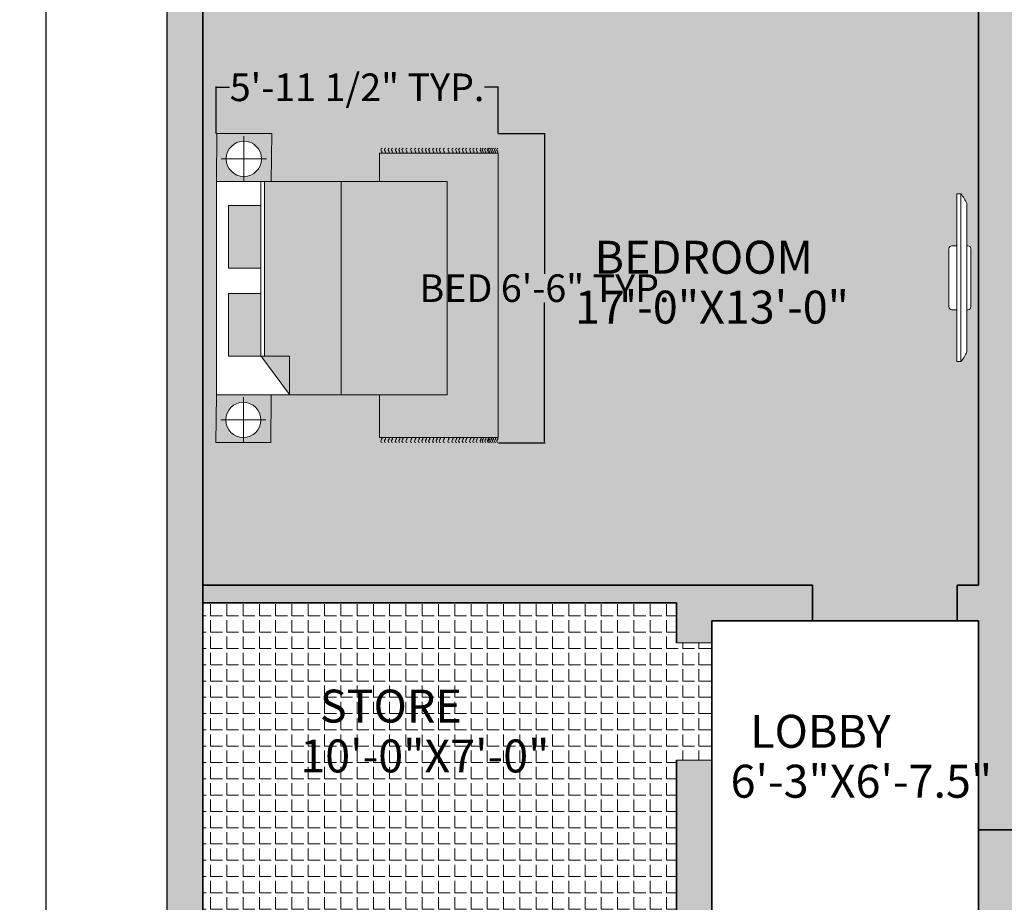
# Model space of a CAD drawing. Units: inches. Extents: x 1884 to 2398, y 474 to 1488.
# Tile 35 of 39: x 1915 to 2165, y 1087 to 1310. Entities that reach past the tile are written whole.
import ezdxf

# ---------------------------------------------------------------- set-up
doc = ezdxf.new("R2010")
doc.units = ezdxf.units.IN
doc.header["$MEASUREMENT"] = 0
doc.linetypes.add('ACAD_ISO02W100', pattern=[15, 12, -3])
for name, color, linetype, lineweight in [('A-ANNO-DIMS', 2, 'Continuous', 18), ('A-AREA-IDEN', 7, 'Continuous', 18), ('A-EQPM', 8, 'Continuous', 18), ('A-FLOR-OVHD', 8, 'ACAD_ISO02W100', 18), ('A-FLOR-PATT', 254, 'Continuous', 13), ('A-FURN-PATT', 253, 'Continuous', 13), ('A-WALL-PATT', 250, 'Continuous', 13), ('C-PROP', 7, 'Continuous', 30), ('furniture', 8, 'Continuous', 18), ('walls', 7, 'Continuous', 35)]:
    doc.layers.add(name, color=color, linetype=linetype, lineweight=lineweight)
doc.layers.add('A-FLOR-CASE-PATT', color=251, linetype='Continuous', lineweight=13, true_color=0x636466)
doc.styles.get("Standard").update_dxf_attribs({"font": 'arial.ttf'})
doc.dimstyles.get("Standard").update_dxf_attribs({"dimtxt": 7, "dimasz": 0.18, "dimexe": 0.18, "dimexo": 0.0625, "dimgap": 0.09, "dimtad": 0, "dimtih": 1, "dimtoh": 1, "dimzin": 0, "dimdsep": 46, "dimlunit": 3, "dimtxsty": 'Standard', "dimcen": 0.09, "dimadec": 0, "dimazin": 0, "dimtfac": 1, "dimtofl": 0, "dimtmove": 0, "dimatfit": 3, "dimfxl": 1, "dimtolj": 1, "dimtzin": 0, "dimarcsym": 0})

# ---------------------------------------------------------------- blocks, each defined once
blk = doc.blocks.new('*D2')
at = {"layer": 'A-ANNO-DIMS', "color": 0, "lineweight": -2, "transparency": 16777216}
for p, q in [((1920.51, 1406.88), (1921.96, 1406.88)), ((1921.78, 1406.7), (1921.78, 972.55)), ((1921.78, 531.06), (1921.78, 965.22)), ((1920.51, 530.88), (1921.96, 530.88))]:
    blk.add_line(p, q, dxfattribs=at)
at = {"layer": 'A-ANNO-DIMS', "color": 0, "lineweight": 100, "transparency": 16777216}
for points in [[(1921.75, 1406.7), (1921.81, 1406.7), (1921.78, 1406.88)], [(1921.75, 531.06), (1921.81, 531.06), (1921.78, 530.88)]]:
    blk.add_solid(points, dxfattribs=at)
at = {"layer": 'Defpoints', "color": 0, "lineweight": 100, "transparency": 16777216}
for p in [(1920.45, 1406.88), (1920.45, 530.88), (1921.78, 530.88)]:
    blk.add_point(p, dxfattribs=at)
at = {"layer": 'A-ANNO-DIMS', "color": 0, "transparency": 16777216, "insert": (1921.78, 968.88), "char_height": 7, "attachment_point": 5}
blk.add_mtext("\\A1;73'", dxfattribs=at)
blk = doc.blocks.new('CARPET')
at = {"layer": 'furniture'}
for p, q in [((-51.53, -98.11), (-51.53, -55.12)), ((-51.53, -55.12), (-41.27, -55.12)), ((36, -55.12), (51.55, -55.12)), ((51.55, -55.12), (51.55, -98.11)), ((51.55, -98.11), (-51.53, -98.11))]:
    blk.add_line(p, q, dxfattribs=at)
for points, knots in [([(-53.37, -55.99), (-53.22, -55.8), (-52.9, -55.41), (-52.34, -55.8), (-51.89, -56.08), (-51.65, -55.91), (-51.53, -55.83)], [0, 0, 0, 0, 0.653278, 1.290138, 1.740457, 2.114451, 2.114451, 2.114451, 2.114451]), ([(-53.37, -57.26), (-53.22, -57.07), (-52.9, -56.67), (-52.34, -57.07), (-51.89, -57.35), (-51.65, -57.17), (-51.53, -57.1)], [0, 0, 0, 0, 0.653278, 1.290138, 1.740457, 2.114451, 2.114451, 2.114451, 2.114451]), ([(53.37, -55.99), (53.22, -55.8), (52.9, -55.41), (52.34, -55.8), (51.89, -56.08), (51.65, -55.91), (51.53, -55.83)], [0, 0, 0, 0, 0.653278, 1.290138, 1.740457, 2.114451, 2.114451, 2.114451, 2.114451]), ([(53.37, -57.26), (53.22, -57.07), (52.9, -56.67), (52.34, -57.07), (51.89, -57.35), (51.65, -57.17), (51.53, -57.1)], [0, 0, 0, 0, 0.653278, 1.290138, 1.740457, 2.114451, 2.114451, 2.114451, 2.114451]), ([(-53.37, -58.59), (-53.22, -58.4), (-52.9, -58.01), (-52.34, -58.4), (-51.89, -58.68), (-51.65, -58.5), (-51.53, -58.43)], [0, 0, 0, 0, 0.653278, 1.290138, 1.740457, 2.114451, 2.114451, 2.114451, 2.114451]), ([(-53.37, -59.78), (-53.22, -59.58), (-52.9, -59.19), (-52.34, -59.58), (-51.89, -59.86), (-51.65, -59.69), (-51.53, -59.61)], [0, 0, 0, 0, 0.653278, 1.290138, 1.740457, 2.114451, 2.114451, 2.114451, 2.114451]), ([(53.37, -58.59), (53.22, -58.4), (52.9, -58.01), (52.34, -58.4), (51.89, -58.68), (51.65, -58.5), (51.53, -58.43)], [0, 0, 0, 0, 0.653278, 1.290138, 1.740457, 2.114451, 2.114451, 2.114451, 2.114451]), ([(53.37, -59.78), (53.22, -59.58), (52.9, -59.19), (52.34, -59.58), (51.89, -59.86), (51.65, -59.69), (51.53, -59.61)], [0, 0, 0, 0, 0.653278, 1.290138, 1.740457, 2.114451, 2.114451, 2.114451, 2.114451]), ([(-53.37, -61.22), (-53.22, -61.02), (-52.9, -60.63), (-52.34, -61.02), (-51.89, -61.3), (-51.65, -61.13), (-51.53, -61.05)], [0, 0, 0, 0, 0.653278, 1.290138, 1.740457, 2.114451, 2.114451, 2.114451, 2.114451]), ([(-53.37, -62.44), (-53.22, -62.25), (-52.9, -61.86), (-52.34, -62.25), (-51.89, -62.53), (-51.65, -62.36), (-51.53, -62.28)], [0, 0, 0, 0, 0.653278, 1.290138, 1.740457, 2.114451, 2.114451, 2.114451, 2.114451]), ([(-53.37, -63.63), (-53.22, -63.43), (-52.9, -63.04), (-52.34, -63.43), (-51.89, -63.72), (-51.65, -63.54), (-51.53, -63.46)], [0, 0, 0, 0, 0.653278, 1.290138, 1.740457, 2.114451, 2.114451, 2.114451, 2.114451]), ([(53.37, -61.22), (53.22, -61.02), (52.9, -60.63), (52.34, -61.02), (51.89, -61.3), (51.65, -61.13), (51.53, -61.05)], [0, 0, 0, 0, 0.653278, 1.290138, 1.740457, 2.114451, 2.114451, 2.114451, 2.114451]), ([(53.37, -62.44), (53.22, -62.25), (52.9, -61.86), (52.34, -62.25), (51.89, -62.53), (51.65, -62.36), (51.53, -62.28)], [0, 0, 0, 0, 0.653278, 1.290138, 1.740457, 2.114451, 2.114451, 2.114451, 2.114451]), ([(53.37, -63.63), (53.22, -63.43), (52.9, -63.04), (52.34, -63.43), (51.89, -63.72), (51.65, -63.54), (51.53, -63.46)], [0, 0, 0, 0, 0.653278, 1.290138, 1.740457, 2.114451, 2.114451, 2.114451, 2.114451]), ([(-53.37, -65.07), (-53.22, -64.87), (-52.9, -64.48), (-52.34, -64.87), (-51.89, -65.15), (-51.65, -64.98), (-51.53, -64.9)], [0, 0, 0, 0, 0.653278, 1.290138, 1.740457, 2.114451, 2.114451, 2.114451, 2.114451]), ([(-53.37, -66.76), (-53.22, -66.56), (-52.9, -66.17), (-52.34, -66.56), (-51.89, -66.84), (-51.65, -66.67), (-51.53, -66.59)], [0, 0, 0, 0, 0.653278, 1.290138, 1.740457, 2.114451, 2.114451, 2.114451, 2.114451]), ([(-53.37, -68.2), (-53.22, -68), (-52.9, -67.61), (-52.34, -68), (-51.89, -68.28), (-51.65, -68.11), (-51.53, -68.03)], [0, 0, 0, 0, 0.653278, 1.290138, 1.740457, 2.114451, 2.114451, 2.114451, 2.114451]), ([(53.37, -65.07), (53.22, -64.87), (52.9, -64.48), (52.34, -64.87), (51.89, -65.15), (51.65, -64.98), (51.53, -64.9)], [0, 0, 0, 0, 0.653278, 1.290138, 1.740457, 2.114451, 2.114451, 2.114451, 2.114451]), ([(53.37, -66.76), (53.22, -66.56), (52.9, -66.17), (52.34, -66.56), (51.89, -66.84), (51.65, -66.67), (51.53, -66.59)], [0, 0, 0, 0, 0.653278, 1.290138, 1.740457, 2.114451, 2.114451, 2.114451, 2.114451]), ([(53.37, -68.2), (53.22, -68), (52.9, -67.61), (52.34, -68), (51.89, -68.28), (51.65, -68.11), (51.53, -68.03)], [0, 0, 0, 0, 0.653278, 1.290138, 1.740457, 2.114451, 2.114451, 2.114451, 2.114451]), ([(-53.37, -69.53), (-53.22, -69.33), (-52.9, -68.94), (-52.34, -69.33), (-51.89, -69.61), (-51.65, -69.44), (-51.53, -69.36)], [0, 0, 0, 0, 0.653278, 1.290138, 1.740457, 2.114451, 2.114451, 2.114451, 2.114451]), ([(-53.37, -70.79), (-53.22, -70.6), (-52.9, -70.21), (-52.34, -70.6), (-51.89, -70.88), (-51.65, -70.7), (-51.53, -70.63)], [0, 0, 0, 0, 0.653278, 1.290138, 1.740457, 2.114451, 2.114451, 2.114451, 2.114451]), ([(53.37, -69.53), (53.22, -69.33), (52.9, -68.94), (52.34, -69.33), (51.89, -69.61), (51.65, -69.44), (51.53, -69.36)], [0, 0, 0, 0, 0.653278, 1.290138, 1.740457, 2.114451, 2.114451, 2.114451, 2.114451]), ([(53.37, -70.79), (53.22, -70.6), (52.9, -70.21), (52.34, -70.6), (51.89, -70.88), (51.65, -70.7), (51.53, -70.63)], [0, 0, 0, 0, 0.653278, 1.290138, 1.740457, 2.114451, 2.114451, 2.114451, 2.114451]), ([(-53.37, -72.12), (-53.22, -71.93), (-52.9, -71.54), (-52.34, -71.93), (-51.89, -72.21), (-51.65, -72.04), (-51.53, -71.96)], [0, 0, 0, 0, 0.653278, 1.290138, 1.740457, 2.114451, 2.114451, 2.114451, 2.114451]), ([(-53.37, -73.31), (-53.22, -73.11), (-52.9, -72.72), (-52.34, -73.11), (-51.89, -73.4), (-51.65, -73.22), (-51.53, -73.14)], [0, 0, 0, 0, 0.653278, 1.290138, 1.740457, 2.114451, 2.114451, 2.114451, 2.114451]), ([(-53.37, -74.75), (-53.22, -74.55), (-52.9, -74.16), (-52.34, -74.55), (-51.89, -74.83), (-51.65, -74.66), (-51.53, -74.58)], [0, 0, 0, 0, 0.653278, 1.290138, 1.740457, 2.114451, 2.114451, 2.114451, 2.114451]), ([(53.37, -72.12), (53.22, -71.93), (52.9, -71.54), (52.34, -71.93), (51.89, -72.21), (51.65, -72.04), (51.53, -71.96)], [0, 0, 0, 0, 0.653278, 1.290138, 1.740457, 2.114451, 2.114451, 2.114451, 2.114451]), ([(53.37, -73.31), (53.22, -73.11), (52.9, -72.72), (52.34, -73.11), (51.89, -73.4), (51.65, -73.22), (51.53, -73.14)], [0, 0, 0, 0, 0.653278, 1.290138, 1.740457, 2.114451, 2.114451, 2.114451, 2.114451]), ([(53.37, -74.75), (53.22, -74.55), (52.9, -74.16), (52.34, -74.55), (51.89, -74.83), (51.65, -74.66), (51.53, -74.58)], [0, 0, 0, 0, 0.653278, 1.290138, 1.740457, 2.114451, 2.114451, 2.114451, 2.114451]), ([(-53.37, -75.98), (-53.22, -75.78), (-52.9, -75.39), (-52.34, -75.78), (-51.89, -76.06), (-51.65, -75.89), (-51.53, -75.81)], [0, 0, 0, 0, 0.653278, 1.290138, 1.740457, 2.114451, 2.114451, 2.114451, 2.114451]), ([(-53.37, -77.16), (-53.22, -76.96), (-52.9, -76.57), (-52.34, -76.96), (-51.89, -77.25), (-51.65, -77.07), (-51.53, -76.99)], [0, 0, 0, 0, 0.653278, 1.290138, 1.740457, 2.114451, 2.114451, 2.114451, 2.114451]), ([(-53.37, -78.6), (-53.22, -78.4), (-52.9, -78.01), (-52.34, -78.4), (-51.89, -78.68), (-51.65, -78.51), (-51.53, -78.43)], [0, 0, 0, 0, 0.653278, 1.290138, 1.740457, 2.114451, 2.114451, 2.114451, 2.114451]), ([(53.37, -75.98), (53.22, -75.78), (52.9, -75.39), (52.34, -75.78), (51.89, -76.06), (51.65, -75.89), (51.53, -75.81)], [0, 0, 0, 0, 0.653278, 1.290138, 1.740457, 2.114451, 2.114451, 2.114451, 2.114451]), ([(53.37, -77.16), (53.22, -76.96), (52.9, -76.57), (52.34, -76.96), (51.89, -77.25), (51.65, -77.07), (51.53, -76.99)], [0, 0, 0, 0, 0.653278, 1.290138, 1.740457, 2.114451, 2.114451, 2.114451, 2.114451]), ([(53.37, -78.6), (53.22, -78.4), (52.9, -78.01), (52.34, -78.4), (51.89, -78.68), (51.65, -78.51), (51.53, -78.43)], [0, 0, 0, 0, 0.653278, 1.290138, 1.740457, 2.114451, 2.114451, 2.114451, 2.114451]), ([(-53.37, -80.29), (-53.22, -80.09), (-52.9, -79.7), (-52.34, -80.09), (-51.89, -80.37), (-51.65, -80.2), (-51.53, -80.12)], [0, 0, 0, 0, 0.653278, 1.290138, 1.740457, 2.114451, 2.114451, 2.114451, 2.114451]), ([(-53.37, -81.73), (-53.22, -81.53), (-52.9, -81.14), (-52.34, -81.53), (-51.89, -81.81), (-51.65, -81.64), (-51.53, -81.56)], [0, 0, 0, 0, 0.653278, 1.290138, 1.740457, 2.114451, 2.114451, 2.114451, 2.114451]), ([(53.37, -80.29), (53.22, -80.09), (52.9, -79.7), (52.34, -80.09), (51.89, -80.37), (51.65, -80.2), (51.53, -80.12)], [0, 0, 0, 0, 0.653278, 1.290138, 1.740457, 2.114451, 2.114451, 2.114451, 2.114451]), ([(53.37, -81.73), (53.22, -81.53), (52.9, -81.14), (52.34, -81.53), (51.89, -81.81), (51.65, -81.64), (51.53, -81.56)], [0, 0, 0, 0, 0.653278, 1.290138, 1.740457, 2.114451, 2.114451, 2.114451, 2.114451]), ([(-53.37, -83.06), (-53.22, -82.86), (-52.9, -82.47), (-52.34, -82.86), (-51.89, -83.14), (-51.65, -82.97), (-51.53, -82.89)], [0, 0, 0, 0, 0.653278, 1.290138, 1.740457, 2.114451, 2.114451, 2.114451, 2.114451]), ([(-53.37, -84.18), (-53.22, -83.99), (-52.9, -83.6), (-52.34, -83.99), (-51.89, -84.27), (-51.65, -84.09), (-51.53, -84.02)], [0, 0, 0, 0, 0.653278, 1.290138, 1.740457, 2.114451, 2.114451, 2.114451, 2.114451]), ([(-53.37, -85.51), (-53.22, -85.32), (-52.9, -84.93), (-52.34, -85.32), (-51.89, -85.6), (-51.65, -85.42), (-51.53, -85.35)], [0, 0, 0, 0, 0.653278, 1.290138, 1.740457, 2.114451, 2.114451, 2.114451, 2.114451]), ([(53.37, -83.06), (53.22, -82.86), (52.9, -82.47), (52.34, -82.86), (51.89, -83.14), (51.65, -82.97), (51.53, -82.89)], [0, 0, 0, 0, 0.653278, 1.290138, 1.740457, 2.114451, 2.114451, 2.114451, 2.114451]), ([(53.37, -84.18), (53.22, -83.99), (52.9, -83.6), (52.34, -83.99), (51.89, -84.27), (51.65, -84.09), (51.53, -84.02)], [0, 0, 0, 0, 0.653278, 1.290138, 1.740457, 2.114451, 2.114451, 2.114451, 2.114451]), ([(53.37, -85.51), (53.22, -85.32), (52.9, -84.93), (52.34, -85.32), (51.89, -85.6), (51.65, -85.42), (51.53, -85.35)], [0, 0, 0, 0, 0.653278, 1.290138, 1.740457, 2.114451, 2.114451, 2.114451, 2.114451]), ([(-53.37, -86.7), (-53.22, -86.5), (-52.9, -86.11), (-52.34, -86.5), (-51.89, -86.78), (-51.65, -86.61), (-51.53, -86.53)], [0, 0, 0, 0, 0.653278, 1.290138, 1.740457, 2.114451, 2.114451, 2.114451, 2.114451]), ([(-53.37, -88.14), (-53.22, -87.94), (-52.9, -87.55), (-52.34, -87.94), (-51.89, -88.22), (-51.65, -88.05), (-51.53, -87.97)], [0, 0, 0, 0, 0.653278, 1.290138, 1.740457, 2.114451, 2.114451, 2.114451, 2.114451]), ([(-53.37, -89.36), (-53.22, -89.17), (-52.9, -88.78), (-52.34, -89.17), (-51.89, -89.45), (-51.65, -89.28), (-51.53, -89.2)], [0, 0, 0, 0, 0.653278, 1.290138, 1.740457, 2.114451, 2.114451, 2.114451, 2.114451]), ([(53.37, -86.7), (53.22, -86.5), (52.9, -86.11), (52.34, -86.5), (51.89, -86.78), (51.65, -86.61), (51.53, -86.53)], [0, 0, 0, 0, 0.653278, 1.290138, 1.740457, 2.114451, 2.114451, 2.114451, 2.114451]), ([(53.37, -88.14), (53.22, -87.94), (52.9, -87.55), (52.34, -87.94), (51.89, -88.22), (51.65, -88.05), (51.53, -87.97)], [0, 0, 0, 0, 0.653278, 1.290138, 1.740457, 2.114451, 2.114451, 2.114451, 2.114451]), ([(53.37, -89.36), (53.22, -89.17), (52.9, -88.78), (52.34, -89.17), (51.89, -89.45), (51.65, -89.28), (51.53, -89.2)], [0, 0, 0, 0, 0.653278, 1.290138, 1.740457, 2.114451, 2.114451, 2.114451, 2.114451]), ([(-53.37, -90.55), (-53.22, -90.35), (-52.9, -89.96), (-52.34, -90.35), (-51.89, -90.64), (-51.65, -90.46), (-51.53, -90.38)], [0, 0, 0, 0, 0.653278, 1.290138, 1.740457, 2.114451, 2.114451, 2.114451, 2.114451]), ([(-53.37, -91.99), (-53.22, -91.79), (-52.9, -91.4), (-52.34, -91.79), (-51.89, -92.07), (-51.65, -91.9), (-51.53, -91.82)], [0, 0, 0, 0, 0.653278, 1.290138, 1.740457, 2.114451, 2.114451, 2.114451, 2.114451]), ([(-53.37, -92.69), (-53.22, -92.48), (-52.9, -92.08), (-52.35, -92.49), (-51.89, -92.77), (-51.65, -92.6), (-51.53, -92.52)], [0, 0, 0, 0, 0.663904, 1.307406, 1.757725, 2.131719, 2.131719, 2.131719, 2.131719]), ([(53.37, -90.55), (53.22, -90.35), (52.9, -89.96), (52.34, -90.35), (51.9, -90.63), (51.66, -90.47), (51.55, -90.4)], [0, 0, 0, 0, 0.653278, 1.290138, 1.740457, 2.0926, 2.0926, 2.0926, 2.0926]), ([(53.37, -91.99), (53.22, -91.79), (52.9, -91.4), (52.34, -91.79), (51.9, -92.07), (51.66, -91.91), (51.55, -91.83)], [0, 0, 0, 0, 0.653278, 1.290138, 1.740457, 2.0926, 2.0926, 2.0926, 2.0926]), ([(53.37, -92.69), (53.22, -92.49), (52.9, -92.09), (52.34, -92.49), (51.9, -92.77), (51.66, -92.61), (51.55, -92.53)], [0, 0, 0, 0, 0.656792, 1.295826, 1.746145, 2.098292, 2.098292, 2.098292, 2.098292]), ([(-53.37, -93.61), (-53.22, -93.42), (-52.9, -93.03), (-52.34, -93.42), (-51.89, -93.7), (-51.65, -93.52), (-51.53, -93.45)], [0, 0, 0, 0, 0.653278, 1.290138, 1.740457, 2.114451, 2.114451, 2.114451, 2.114451]), ([(-53.37, -94.55), (-53.22, -94.35), (-52.9, -93.96), (-52.34, -94.35), (-51.89, -94.63), (-51.65, -94.46), (-51.53, -94.38)], [0, 0, 0, 0, 0.653278, 1.290138, 1.740457, 2.114451, 2.114451, 2.114451, 2.114451]), ([(-53.37, -95.05), (-53.22, -94.85), (-52.9, -94.46), (-52.34, -94.85), (-51.89, -95.14), (-51.65, -94.96), (-51.53, -94.88)], [0, 0, 0, 0, 0.653278, 1.290138, 1.740457, 2.114451, 2.114451, 2.114451, 2.114451]), ([(-53.37, -95.73), (-53.22, -95.54), (-52.9, -95.15), (-52.34, -95.54), (-51.89, -95.82), (-51.65, -95.65), (-51.53, -95.57)], [0, 0, 0, 0, 0.653278, 1.290138, 1.740457, 2.114451, 2.114451, 2.114451, 2.114451]), ([(-53.37, -96.38), (-53.22, -96.18), (-52.9, -95.79), (-52.34, -96.18), (-51.89, -96.47), (-51.65, -96.29), (-51.53, -96.21)], [0, 0, 0, 0, 0.653278, 1.290138, 1.740457, 2.114451, 2.114451, 2.114451, 2.114451]), ([(53.37, -95.78), (53.22, -95.58), (52.9, -95.19), (52.34, -95.58), (51.89, -95.86), (51.65, -95.69), (51.53, -95.61)], [0, 0, 0, 0, 0.653278, 1.290138, 1.740457, 2.114451, 2.114451, 2.114451, 2.114451]), ([(53.37, -96.43), (53.22, -96.23), (52.9, -95.84), (52.34, -96.23), (51.89, -96.51), (51.65, -96.34), (51.53, -96.26)], [0, 0, 0, 0, 0.653278, 1.290138, 1.740457, 2.114451, 2.114451, 2.114451, 2.114451]), ([(53.37, -93.66), (53.22, -93.46), (52.9, -93.07), (52.34, -93.46), (51.9, -93.74), (51.66, -93.58), (51.55, -93.5)], [0, 0, 0, 0, 0.653278, 1.290138, 1.740457, 2.0926, 2.0926, 2.0926, 2.0926]), ([(53.37, -94.59), (53.22, -94.4), (52.9, -94.01), (52.34, -94.4), (51.9, -94.68), (51.66, -94.51), (51.55, -94.44)], [0, 0, 0, 0, 0.653278, 1.290138, 1.740457, 2.0926, 2.0926, 2.0926, 2.0926]), ([(53.37, -95.1), (53.22, -94.9), (52.9, -94.51), (52.34, -94.9), (51.9, -95.18), (51.66, -95.02), (51.55, -94.94)], [0, 0, 0, 0, 0.653278, 1.290138, 1.740457, 2.0926, 2.0926, 2.0926, 2.0926]), ([(-53.37, -97.17), (-53.22, -96.98), (-52.9, -96.59), (-52.34, -96.98), (-51.89, -97.26), (-51.65, -97.08), (-51.53, -97.01)], [0, 0, 0, 0, 0.653278, 1.290138, 1.740457, 2.114451, 2.114451, 2.114451, 2.114451]), ([(-53.37, -97.99), (-53.22, -97.79), (-52.9, -97.4), (-52.34, -97.79), (-51.89, -98.08), (-51.65, -97.9), (-51.53, -97.82)], [0, 0, 0, 0, 0.653278, 1.290138, 1.740457, 2.114451, 2.114451, 2.114451, 2.114451]), ([(53.37, -97.22), (53.22, -97.02), (52.9, -96.63), (52.34, -97.02), (51.89, -97.3), (51.65, -97.13), (51.53, -97.05)], [0, 0, 0, 0, 0.653278, 1.290138, 1.740457, 2.114451, 2.114451, 2.114451, 2.114451]), ([(53.37, -97.99), (53.22, -97.79), (52.9, -97.4), (52.34, -97.79), (51.89, -98.08), (51.65, -97.9), (51.53, -97.82)], [0, 0, 0, 0, 0.653278, 1.290138, 1.740457, 2.114451, 2.114451, 2.114451, 2.114451])]:
    blk.add_open_spline(points, degree=3, knots=knots, dxfattribs=at)
blk = doc.blocks.new('A$C58D270C6')
at = {"layer": 'furniture'}
for p, q in [((9.09, 124.13), (9.09, 108.87)), ((1.46, 116.5), (16.73, 116.5)), ((14.97, 94.84), (24.62, 107.92)), ((24.62, 94.93), (24.62, 107.92)), ((42.08, 108), (42.08, 36)), ((14.97, 94.93), (24.62, 94.93)), ((14.97, 94.84), (14.97, 36)), ((16.22, 94.93), (16.22, 36)), ((9.25, 36), (9.25, 20.74)), ((1.62, 28.37), (16.88, 28.37))]:
    blk.add_line(p, q, dxfattribs=at)
for points in [[(18.5, 108), (18.34, 124.13), (-0.16, 124.13), (0, 108)], [(0, 108), (77.91, 108), (77.91, 36), (0, 36)], [(4.09, 94.93), (14.97, 94.93), (14.97, 73.83), (4.09, 73.83)], [(4.09, 65.23), (14.97, 65.23), (14.97, 44.13), (4.09, 44.13)], [(18.65, 19.87), (18.5, 36), (0, 36), (0.16, 19.87)]]:
    blk.add_lwpolyline(points, close=True, dxfattribs=at)
for centre in [(9.09, 116.5), (9.25, 28.37)]:
    blk.add_circle(centre, 5.95, dxfattribs=at)
at = {"layer": 'furniture', "xscale": 0.9312884925094044, "yscale": 0.9312884925094044, "zscale": 0.9312884925094044, "rotation": 90}
blk.add_blockref('CARPET', (3.79, 74.47), dxfattribs=at)
blk = doc.blocks.new('PLASMA-LARGE')
at = {"layer": 'furniture'}
for p, q in [((-7.26, 0), (7.26, 0)), ((-18.61, -1), (18.61, -1)), ((-8, -1), (-8, -0.74)), ((8, -1), (8, -0.74)), ((-21, -2.5), (21, -2.5)), ((-21, -2.5), (-21, -3.5)), ((-21, -3.5), (21, -3.5)), ((-8, -3.5), (-8, -4.76)), ((8, -3.5), (8, -4.76)), ((21, -2.5), (21, -3.5)), ((-7.26, -5.5), (7.26, -5.5))]:
    blk.add_line(p, q, dxfattribs=at)
for centre, radius, start, end in [((-7.26, -0.74), 0.744, 90, 180), ((7.26, -0.74), 0.744, 0, 90), ((-13.97, -11.05), 11.07, 114.7602, 129.4175), ((13.97, -11.05), 11.07, 50.5825, 65.2398), ((-7.26, -4.76), 0.744, 180, 270), ((7.26, -4.76), 0.744, 270, 0)]:
    blk.add_arc(centre, radius, start, end, dxfattribs=at)
blk = doc.blocks.new('*D25')
at = {"layer": 'A-ANNO-DIMS', "color": 0, "lineweight": -2, "transparency": 16777216}
for p, q in [((2036.44, 1281.21), (2048.29, 1281.21)), ((2048.11, 1281.03), (2048.11, 1245.75)), ((2048.11, 1203.15), (2048.11, 1238.43)), ((2036.44, 1202.97), (2048.29, 1202.97))]:
    blk.add_line(p, q, dxfattribs=at)
at = {"layer": 'A-ANNO-DIMS', "color": 0, "lineweight": 100, "transparency": 16777216}
for points in [[(2048.08, 1281.03), (2048.14, 1281.03), (2048.11, 1281.21)], [(2048.08, 1203.15), (2048.14, 1203.15), (2048.11, 1202.97)]]:
    blk.add_solid(points, dxfattribs=at)
at = {"layer": 'Defpoints', "color": 0, "lineweight": 100, "transparency": 16777216}
for p in [(2036.38, 1281.21), (2036.38, 1202.97), (2048.11, 1202.97)]:
    blk.add_point(p, dxfattribs=at)
at = {"layer": 'A-ANNO-DIMS', "color": 0, "transparency": 16777216, "insert": (2048.11, 1242.09), "char_height": 7, "attachment_point": 5}
blk.add_mtext('\\A1;BED 6\'-6" TYP.', dxfattribs=at)
blk = doc.blocks.new('*D26')
at = {"layer": 'A-ANNO-DIMS', "color": 0, "lineweight": -2, "transparency": 16777216}
for p, q in [((1964.89, 1281.27), (1964.89, 1293.12)), ((1965.07, 1292.94), (1968.33, 1292.94)), ((2036.2, 1292.94), (2032.93, 1292.94)), ((2036.38, 1281.27), (2036.38, 1293.12))]:
    blk.add_line(p, q, dxfattribs=at)
at = {"layer": 'A-ANNO-DIMS', "color": 0, "lineweight": 100, "transparency": 16777216}
for points in [[(1965.07, 1292.97), (1965.07, 1292.91), (1964.89, 1292.94)], [(2036.2, 1292.97), (2036.2, 1292.91), (2036.38, 1292.94)]]:
    blk.add_solid(points, dxfattribs=at)
at = {"layer": 'Defpoints', "color": 0, "lineweight": 100, "transparency": 16777216}
for p in [(2036.38, 1292.94), (1964.89, 1281.21), (2036.38, 1281.21)]:
    blk.add_point(p, dxfattribs=at)
at = {"layer": 'A-ANNO-DIMS', "color": 0, "transparency": 16777216, "insert": (2000.63, 1292.94), "char_height": 7, "attachment_point": 5}
blk.add_mtext('\\A1;5\'-11 1/2" TYP.', dxfattribs=at)

msp = doc.modelspace()

# ---------------------------------------------------------------- hatches: boundary and pattern name
at = {"layer": 'A-FLOR-CASE-PATT'}
h = msp.add_hatch(color=256, dxfattribs=at)
h.dxf.hatch_style = 1
h.paths.add_polyline_path([(2143.18, 1275.904), (2158.076, 1275.904), (2158.076, 1211.461), (2143.18, 1211.461)])
h.paths.add_polyline_path([(2152.587, 1223.485), (2153.598, 1223.485, 0.0640419), (2155.115, 1225.904), (2155.115, 1236.632), (2155.374, 1236.632, 0.4142136), (2156.126, 1237.385), (2156.126, 1252.06, 0.4142136), (2155.374, 1252.813), (2155.115, 1252.813), (2155.115, 1263.54, 0.0640419), (2153.598, 1265.959), (2152.587, 1265.959), (2152.587, 1252.813), (2151.317, 1252.813, 0.4142136), (2150.564, 1252.06), (2150.564, 1237.385, 0.4142136), (2151.317, 1236.632), (2152.587, 1236.632)], flags=16)
at = {"layer": 'A-FLOR-PATT'}
h = msp.add_hatch(color=256, dxfattribs=at)
h.dxf.hatch_style = 1
h.paths.add_polyline_path([(2117.529, 815.801), (2126.529, 815.801), (2126.529, 880.382), (2117.529, 880.382), (2117.529, 892.385), (1961.529, 892.385), (1961.529, 756.915), (1964.529, 756.915), (1964.529, 759.915), (1995.529, 759.915), (1995.529, 753.915), (1972.862, 753.915), (1967.529, 756.915), (1967.529, 654.915), (1972.862, 657.915), (1995.529, 657.915), (1995.529, 651.915), (1964.529, 651.915), (1964.529, 654.915), (1961.529, 654.915), (1961.529, 640.385), (2117.529, 640.385), (2117.529, 646.578), (2126.529, 646.578), (2126.529, 676.183), (2117.529, 676.183)])
h.paths.add_polyline_path([(2012.246, 808.929), (2012.05, 810.185), (2032.542, 810.185), (2032.346, 808.929)], flags=16)
h.paths.add_polyline_path([(2010.381, 820.864), (1994.658, 820.864), (1994.658, 831.561), (1984.608, 833.132), (1984.608, 853.821), (1994.658, 855.391), (1994.658, 866.089), (2010.381, 866.089), (2011.951, 876.139), (2032.64, 876.139), (2034.211, 866.089), (2045.556, 866.089), (2047.127, 876.139), (2067.816, 876.139), (2069.386, 866.089), (2085.109, 866.089), (2085.109, 855.391), (2095.159, 853.821), (2095.159, 833.132), (2085.109, 831.561), (2085.109, 820.864), (2069.386, 820.864), (2067.816, 810.814), (2047.127, 810.814), (2045.556, 820.864), (2034.211, 820.864), (2032.64, 810.814), (2011.951, 810.814)], flags=16)
h.paths.add_polyline_path([(1982.724, 833.426), (1982.724, 853.526), (1983.98, 853.723), (1983.98, 833.23)], flags=16)
h.paths.add_polyline_path([(1994.529, 753.54), (1994.529, 658.29), (1973.529, 658.29), (1973.529, 753.54)], flags=16)
h.paths.add_polyline_path([(2084.486, 843.527), (2084.592, 843.502), (2084.681, 843.487), (2084.813, 843.477), (2084.913, 843.477), (2084.669, 843.482), (2084.336, 843.565), (2084.116, 843.617), (2083.8, 843.686), (2083.105, 843.827), (2082.836, 843.874), (2083.604, 843.729), (2084.206, 843.597)], flags=0)
h.paths.add_polyline_path([(2047.421, 808.929), (2047.225, 810.185), (2067.718, 810.185), (2067.521, 808.929)], flags=16)
h.paths.add_polyline_path([(2066.01, 849.505), (2066.429, 849.687), (2066.798, 849.882), (2067.129, 850.085), (2067.43, 850.293), (2067.711, 850.502), (2068.176, 850.856), (2068.689, 851.205), (2069.305, 851.531), (2070.015, 851.784), (2070.844, 851.944), (2071.081, 851.956), (2070.629, 851.902), (2070.212, 851.822), (2069.827, 851.717), (2069.471, 851.59), (2069.139, 851.443), (2068.828, 851.279), (2068.534, 851.1), (2068.254, 850.909), (2067.983, 850.709), (2067.502, 850.343), (2066.951, 849.962), (2066.224, 849.579)], flags=0)
h.paths.add_polyline_path([(2059.423, 853.221), (2059.827, 853.278), (2060.171, 853.358), (2060.465, 853.463), (2060.714, 853.589), (2060.926, 853.736), (2061.107, 853.902), (2061.258, 854.086), (2061.377, 854.284), (2061.462, 854.495), (2061.514, 854.715), (2061.53, 854.943), (2061.508, 855.176), (2061.449, 855.411), (2061.352, 855.646), (2061.224, 855.882), (2061.07, 856.117), (2060.9, 856.353), (2060.719, 856.588), (2060.406, 856.993), (2060.103, 857.424), (2059.858, 857.888), (2059.691, 858.467), (2059.836, 859.091), (2060.305, 859.532), (2060.844, 859.798), (2061.513, 859.935), (2062.253, 859.905), (2062.483, 859.849), (2062.078, 859.912), (2061.695, 859.928), (2061.336, 859.899), (2061.005, 859.831), (2060.703, 859.729), (2060.437, 859.597), (2060.208, 859.441), (2060.021, 859.265), (2059.879, 859.075), (2059.785, 858.874), (2059.737, 858.664), (2059.73, 858.447), (2059.761, 858.224), (2059.827, 857.996), (2059.923, 857.765), (2060.047, 857.53), (2060.193, 857.295), (2060.359, 857.06), (2060.537, 856.824), (2060.867, 856.399), (2061.171, 855.978), (2061.422, 855.518), (2061.567, 854.943), (2061.41, 854.272), (2060.947, 853.707), (2060.335, 853.397), (2059.649, 853.236)], flags=0)
h.paths.add_polyline_path([(2050.778, 859.745), (2051.07, 859.87), (2051.295, 860.017), (2051.467, 860.183), (2051.594, 860.365), (2051.679, 860.56), (2051.726, 860.763), (2051.739, 860.971), (2051.722, 861.18), (2051.677, 861.387), (2051.609, 861.587), (2051.521, 861.779), (2051.421, 861.962), (2051.312, 862.138), (2051.203, 862.307), (2050.966, 862.68), (2050.793, 863.193), (2051.021, 863.699), (2051.483, 864.018), (2052.09, 864.138), (2052.773, 864.157), (2053.007, 864.142), (2052.603, 864.152), (2052.258, 864.142), (2051.965, 864.113), (2051.716, 864.064), (2051.504, 863.995), (2051.322, 863.907), (2051.17, 863.802), (2051.048, 863.682), (2050.954, 863.55), (2050.891, 863.408), (2050.856, 863.259), (2050.851, 863.105), (2050.876, 862.948), (2050.929, 862.791), (2051.005, 862.633), (2051.098, 862.472), (2051.203, 862.307), (2051.312, 862.138), (2051.556, 861.742), (2051.751, 861.167), (2051.712, 860.535), (2051.398, 860.085), (2050.949, 859.79)], flags=0)
h.paths.add_polyline_path([(2022.768, 719.264), (2050.461, 719.264), (2050.461, 717.226), (2052.426, 717.226), (2052.426, 715.033), (2050.461, 715.033), (2050.461, 703.738), (2022.768, 703.738)], flags=16)
h.paths.add_polyline_path([(2012.246, 878.023), (2032.346, 878.023), (2032.542, 876.767), (2012.05, 876.767)], flags=16)
h.paths.add_polyline_path([(2035.324, 713.103), (2035.342, 713.294), (2035.192, 713.202)], flags=0)
h.paths.add_polyline_path([(2036.484, 711.63), (2036.583, 711.849), (2036.39, 711.898)], flags=0)
h.paths.add_polyline_path([(2036.074, 712.744), (2035.993, 712.481), (2035.724, 712.516), (2035.794, 712.726)], flags=0)
h.paths.add_polyline_path([(2035.846, 710.909), (2035.753, 710.958), (2035.702, 710.88)], flags=0)
h.paths.add_polyline_path([(2037.818, 712.019), (2037.948, 712.06), (2037.987, 712.161), (2037.815, 712.02)], flags=0)
h.paths.add_polyline_path([(2038.451, 709.517), (2038.464, 709.428), (2038.586, 709.442)], flags=0)
h.paths.add_polyline_path([(2037.805, 709.806), (2037.818, 709.807), (2037.804, 709.823)], flags=0)
h.paths.add_polyline_path([(2036.7, 711.245), (2036.698, 711.236), (2036.813, 711.211)], flags=0)
h.paths.add_polyline_path([(2035.928, 708.897), (2035.668, 708.871), (2035.706, 708.667)], flags=0)
h.paths.add_polyline_path([(2036.414, 710.976), (2035.932, 709.859), (2036.792, 710.484), (2036.5, 710.934)], flags=0)
h.paths.add_polyline_path([(2038.298, 712.115), (2038.499, 712.058), (2038.612, 712.269), (2038.39, 712.332)], flags=0)
h.paths.add_polyline_path([(2047.421, 878.023), (2067.521, 878.023), (2067.718, 876.767), (2047.225, 876.767)], flags=16)
h.paths.add_polyline_path([(2049.647, 705.093, -1), (2048.845, 705.093, -1)], flags=0)
h.paths.add_polyline_path([(2095.787, 853.723), (2097.043, 853.526), (2097.043, 833.426), (2095.787, 833.23)], flags=16)
h.paths.add_polyline_path([(2110.739, 745.339), (2111.75, 745.339, -0.0640419), (2113.267, 742.92), (2113.267, 732.192), (2113.526, 732.192, -0.4142136), (2114.278, 731.439), (2114.278, 716.764, -0.4142136), (2113.526, 716.011), (2113.267, 716.011), (2113.267, 705.284, -0.0640419), (2111.75, 702.864), (2110.739, 702.864), (2110.739, 716.011), (2109.469, 716.011, -0.4142136), (2108.716, 716.764), (2108.716, 731.439, -0.4142136), (2109.469, 732.192), (2110.739, 732.192)], flags=16)
h.paths.add_polyline_path([(1998.045, 668.909), (2002.449, 668.909), (2002.449, 652.273), (2002.724, 652.763), (2002.724, 668.175), (2019.972, 668.175), (2019.972, 652.763), (2020.247, 652.273), (2020.247, 668.909), (2024.651, 668.909), (2029.055, 668.909), (2029.055, 652.273), (2029.33, 652.763), (2029.33, 668.175), (2046.578, 668.175), (2046.578, 652.763), (2046.853, 652.273), (2046.853, 668.909), (2051.257, 668.909), (2051.257, 646.157), (2049.055, 646.157), (2049.055, 643.955), (2026.853, 643.955), (2026.853, 646.157), (2024.651, 646.157), (2022.449, 646.157), (2022.449, 643.955), (2000.247, 643.955), (2000.247, 646.157), (1998.045, 646.157)], flags=16)
h.paths.add_polyline_path([(2342.529, 1247.885), (2265.892, 1247.885), (2230.029, 1247.885), (2209.755, 1247.885), (2168.6, 1247.885), (2168.6, 1104.929), (2158.029, 1104.929), (2158.029, 1079.411), (2168.6, 1079.411), (2168.6, 1062.466), (2342.529, 1062.466), (2342.529, 1093.809)])
h.paths.add_polyline_path([(2215.03, 1153.876), (2215.03, 1164.739), (2187.559, 1164.739), (2187.442, 1152.641), (2173.568, 1152.641), (2173.684, 1164.739), (2173.684, 1218.739), (2173.801, 1230.837), (2187.675, 1230.837), (2187.559, 1218.739), (2215.03, 1218.739), (2215.03, 1225.879), (2245.053, 1225.879), (2245.053, 1153.876)], flags=16)
h.paths.add_polyline_path([(2192.147, 1164.797), (2184.963, 1174.54), (2184.915, 1174.54), (2176.755, 1174.54), (2176.755, 1190.363), (2184.915, 1190.363), (2184.915, 1196.819), (2176.755, 1196.819), (2176.755, 1212.641), (2184.915, 1212.641), (2184.915, 1174.606), (2184.963, 1174.54), (2192.147, 1174.54)], flags=0)
h.paths.add_polyline_path([(2184.971, 1158.364, -1), (2176.039, 1158.364, -1)], flags=0)
h.paths.add_polyline_path([(2335.555, 1161.985), (2335.555, 1175.132), (2334.285, 1175.132, -0.4142136), (2333.533, 1175.885), (2333.533, 1190.56, -0.4142136), (2334.285, 1191.313), (2335.555, 1191.313), (2335.555, 1204.46), (2336.567, 1204.46, -0.0640419), (2338.083, 1202.04), (2338.083, 1191.313), (2338.342, 1191.313, -0.4142136), (2339.095, 1190.56), (2339.095, 1175.885, -0.4142136), (2338.342, 1175.132), (2338.083, 1175.132), (2338.083, 1164.405, -0.0640419), (2336.567, 1161.985)], flags=16)
h.paths.add_polyline_path([(2176.155, 1224.462, -1), (2185.087, 1224.462, -1)], flags=0)
h.paths.add_polyline_path([(2158.029, 1276.197), (2158.029, 1322.885), (2148.233, 1322.885), (2092.029, 1322.885), (1961.529, 1322.885), (1961.529, 1166.885), (2116.005, 1166.885), (2116.005, 1157.885), (2152.638, 1157.885), (2152.638, 1166.885), (2158.029, 1166.885)])
h.paths.add_polyline_path([(2006.352, 1204.245), (2006.352, 1215.108), (1978.881, 1215.108), (1978.764, 1203.01), (1964.89, 1203.01), (1965.006, 1215.108), (1965.006, 1269.108), (1965.123, 1281.207), (1978.997, 1281.207), (1978.881, 1269.108), (2006.352, 1269.108), (2006.352, 1276.248), (2036.375, 1276.248), (2036.375, 1204.245)], flags=16)
h.paths.add_polyline_path([(1983.469, 1215.166), (1976.285, 1224.909), (1976.237, 1224.909), (1968.077, 1224.909), (1968.077, 1240.732), (1976.237, 1240.732), (1976.237, 1247.188), (1968.077, 1247.188), (1968.077, 1263.011), (1976.237, 1263.011), (1976.237, 1224.975), (1976.285, 1224.909), (1983.469, 1224.909)], flags=0)
h.paths.add_polyline_path([(1976.293, 1208.733, -1), (1967.361, 1208.733, -1)], flags=0)
h.paths.add_polyline_path([(1967.477, 1274.832, -1), (1976.41, 1274.832, -1)], flags=0)
h.paths.add_polyline_path([(2152.587, 1223.485), (2152.587, 1236.632), (2151.317, 1236.632, -0.4142136), (2150.564, 1237.385), (2150.564, 1252.06, -0.4142136), (2151.317, 1252.813), (2152.587, 1252.813), (2152.587, 1265.959), (2153.598, 1265.959, -0.0640419), (2155.115, 1263.54), (2155.115, 1252.813), (2155.374, 1252.813, -0.4142136), (2156.126, 1252.06), (2156.126, 1237.385, -0.4142136), (2155.374, 1236.632), (2155.115, 1236.632), (2155.115, 1225.904, -0.0640419), (2153.598, 1223.485)], flags=16)
h.paths.add_polyline_path([(2250.676, 1161.101), (2322.077, 1161.101), (2322.077, 1173.886), (2250.676, 1173.886)], flags=24)
h.paths.add_polyline_path([(2255.61, 1173.712), (2320.136, 1173.712), (2320.136, 1186.659), (2255.61, 1186.659)], flags=24)
h.paths.add_polyline_path([(2053.687, 1230.837), (2125.089, 1230.837), (2125.089, 1243.622), (2053.687, 1243.622)], flags=24)
h.paths.add_polyline_path([(2058.622, 1243.448), (2123.147, 1243.448), (2123.147, 1256.395), (2058.622, 1256.395)], flags=24)
h = msp.add_hatch(dxfattribs=at)
h.set_pattern_fill('ANGLE', color=256, scale=15)
h.set_pattern_definition([(0, (0, 0), (0, 4.125), [3, -1.125]), (90, (0, 0), (-4.125, 3e-16), [3, -1.125])])
h.paths.add_polyline_path([(2081.529, 1122.635), (2090.529, 1122.635), (2090.529, 1152.292), (2081.529, 1152.292), (2081.529, 1162.385), (1961.529, 1162.385), (1961.529, 1078.385), (2081.529, 1078.385)])
at = {"layer": 'A-FURN-PATT'}
h = msp.add_hatch(color=256, dxfattribs=at)
h.dxf.hatch_style = 1
h.paths.add_polyline_path([(1976.41, 1274.832, 1), (1967.477, 1274.832, 0.4142136), (1971.944, 1270.366), (1971.944, 1269.108), (1965.006, 1269.108), (1965.123, 1281.207), (1978.997, 1281.207), (1978.881, 1269.108), (1971.944, 1269.108), (1971.944, 1270.366, 0.4142136)])
h.paths.add_polyline_path([(1967.361, 1208.733, 0.4142136), (1971.827, 1204.267), (1971.827, 1203.01), (1964.89, 1203.01), (1965.006, 1215.108), (1978.881, 1215.108), (1978.764, 1203.01), (1971.827, 1203.01), (1971.827, 1204.267, 0.4142136), (1976.293, 1208.733, 1)])
h.paths.add_polyline_path([(1976.285, 1224.909), (1983.469, 1224.909), (1983.469, 1215.166)])
h = msp.add_hatch(color=256, dxfattribs=at)
h.dxf.hatch_style = 1
h.paths.add_polyline_path([(2023.435, 1269.108), (2006.352, 1269.108), (2006.352, 1276.248), (2036.375, 1276.248), (2036.375, 1204.245), (2006.352, 1204.245), (2006.352, 1215.108), (2023.435, 1215.108)])
h.paths.add_polyline_path([(1996.565, 1269.108), (2023.435, 1269.108), (2023.435, 1215.108), (1996.565, 1215.108)])
h = msp.add_hatch(color=256, dxfattribs=at)
h.dxf.hatch_style = 1
h.paths.add_polyline_path([(1977.169, 1269.108), (1996.565, 1269.108), (1996.565, 1215.108), (1983.512, 1215.108), (1983.469, 1215.166), (1983.469, 1224.909), (1977.169, 1224.909)])
h = msp.add_hatch(color=256, dxfattribs=at)
h.dxf.hatch_style = 1
h.paths.add_polyline_path([(1968.077, 1263.011), (1976.237, 1263.011), (1976.237, 1247.188), (1968.077, 1247.188)])
h.paths.add_polyline_path([(1968.077, 1240.732), (1976.237, 1240.732), (1976.237, 1224.909), (1968.077, 1224.909)])
at = {"layer": 'A-WALL-PATT'}
h = msp.add_hatch(color=256, dxfattribs=at)
h.dxf.hatch_style = 1
h.paths.add_polyline_path([(2092.029, 1406.885), (1952.529, 1406.885), (1952.529, 939.249), (1955.529, 939.249), (1955.529, 1069.385), (1969.695, 1069.385), (1969.695, 1078.385), (1961.529, 1078.385), (1961.529, 1397.885), (2087.529, 1397.885), (2087.529, 1322.885), (2092.029, 1322.885), (2092.029, 1328.623)])
h.paths.add_polyline_path([(2087.529, 1345.919), (2014.612, 1345.919), (2014.612, 1327.385), (2007.132, 1327.385), (2007.132, 1322.885), (2019.112, 1322.885), (2019.112, 1327.385), (2019.112, 1341.419), (2087.529, 1341.419)], flags=17)
h.paths.add_polyline_path([(1965.066, 1327.561), (1961.529, 1327.561), (1961.529, 1322.885), (1965.066, 1322.885)], flags=17)
h.paths.add_polyline_path([(2351.529, 1343.885), (2265.892, 1343.885), (2164.726, 1343.885), (2158.029, 1343.885), (2158.029, 1334.885), (2158.029, 1328.623), (2148.233, 1328.623), (2148.233, 1322.885), (2158.029, 1322.885), (2158.029, 1276.197), (2158.029, 1166.885), (2152.638, 1166.885), (2152.638, 1157.885), (2158.029, 1157.885), (2158.029, 1104.929), (2168.6, 1104.929), (2168.6, 1247.885), (2209.755, 1247.885), (2209.755, 1252.385), (2167.029, 1252.385), (2167.029, 1334.885), (2265.892, 1334.885), (2342.529, 1334.885), (2342.529, 1310.041), (2351.529, 1310.041)])
h.paths.add_polyline_path([(2234.529, 1334.885), (2230.029, 1334.885), (2230.029, 1275.554), (2234.529, 1275.554)], flags=17)
h.paths.add_polyline_path([(2342.529, 1252.385), (2265.892, 1252.385), (2234.529, 1252.385), (2234.529, 1256.117), (2230.029, 1256.117), (2230.029, 1247.885), (2265.892, 1247.885), (2342.529, 1247.885)], flags=17)
h.paths.add_polyline_path([(2351.529, 1276.197), (2351.529, 1293.635), (2342.529, 1293.635), (2342.529, 1252.385), (2342.529, 1225.302), (2346.311, 1225.302), (2351.529, 1225.302)], flags=17)
h.paths.add_polyline_path([(2351.529, 1126.264), (2342.529, 1126.264), (2342.529, 1093.809), (2342.529, 1062.466), (2168.6, 1062.466), (2168.6, 1079.411), (2158.029, 1079.411), (2158.029, 1056.803), (2158.029, 1053.466), (2213.529, 1053.466), (2213.529, 934.675), (2222.529, 934.675), (2222.529, 1057.966), (2342.529, 1057.966), (2342.529, 1027.206), (2345.987, 1027.206), (2351.529, 1027.206)])
h.paths.add_polyline_path([(2116.005, 1166.885), (1961.529, 1166.885), (1961.529, 1162.385), (2081.529, 1162.385), (2081.529, 1152.292), (2090.529, 1152.292), (2090.529, 1157.885), (2116.005, 1157.885)])
h.paths.add_polyline_path([(2090.529, 1122.635), (2081.529, 1122.635), (2081.529, 1078.385), (2000.529, 1078.385), (2000.529, 1069.385), (2000.529, 1034.463), (2003.893, 1034.463), (2009.529, 1034.463), (2009.529, 1069.385), (2090.529, 1069.385)], flags=17)
h.paths.add_polyline_path([(2351.529, 974.676), (2342.529, 974.676), (2342.529, 951.86), (2351.529, 951.86)], flags=17)

# ---------------------------------------------------------------- linework, layer by layer
at = {"layer": 'A-FLOR-OVHD'}
for p, q in [((2081.529, 1152.292), (2090.529, 1152.292)), ((2081.529, 1122.635), (2090.529, 1122.635))]:
    msp.add_line(p, q, dxfattribs=at)
at = {"layer": 'C-PROP'}
msp.add_line((1952.529, 939.249), (1952.529, 1406.885), dxfattribs=at)
at = {"layer": 'walls'}
for p, q in [((1961.529, 1078.385), (1961.529, 1397.885)), ((2158.029, 1276.197), (2158.029, 1322.885)), ((2158.029, 1166.885), (2158.029, 1276.197)), ((1961.529, 1166.885), (2116.005, 1166.885)), ((2116.005, 1157.885), (2116.005, 1166.885)), ((2152.638, 1166.885), (2152.638, 1157.885)), ((2152.638, 1166.885), (2158.029, 1166.885)), ((1961.529, 1162.385), (2081.529, 1162.385)), ((2081.529, 1152.292), (2081.529, 1162.385)), ((2090.529, 1069.385), (2090.529, 1157.885)), ((2090.529, 1157.885), (2158.029, 1157.885)), ((2158.029, 1104.929), (2158.029, 1157.885)), ((2081.529, 1078.385), (2081.529, 1122.635)), ((2168.6, 1104.929), (2158.029, 1104.929)), ((2158.029, 1104.929), (2158.029, 1056.803))]:
    msp.add_line(p, q, dxfattribs=at)

# ---------------------------------------------------------------- block references
at = {"layer": 'A-EQPM', "xscale": -1.011294184530666, "yscale": 1.011294184530666, "zscale": 1.011294184530666, "rotation": 270}
msp.add_blockref('PLASMA-LARGE', (2156.126, 1244.722), dxfattribs=at)
at = {"layer": 'furniture', "xscale": -0.7500000390647866, "yscale": 0.7500000390647866, "zscale": 0.7500000390647866, "rotation": 180}
msp.add_blockref('A$C58D270C6', (1965.006, 1296.108), dxfattribs=at)

# ---------------------------------------------------------------- texts
at = {"layer": 'A-AREA-IDEN'}
for s, height, p in [('BEDROOM', 8.3413, (2060.779, 1245.748)), ('17\'-0"X13\'-0"', 8.34125, (2055.818, 1233.116)), ('STORE', 8.3413, (1991.201, 1132.112)), ('LOBBY', 8.3413, (2100.219, 1125.726)), ('10\'-0"X7\'-0"', 8.34125, (1986.24, 1119.48)), ('6\'-3"X6\'-7.5"', 8.34125, (2095.257, 1113.093))]:
    msp.add_text(s, height=height, dxfattribs=at).set_placement(p)

# ---------------------------------------------------------------- dimensions: what is measured, and where the dimension line sits
at = {"layer": 'A-ANNO-DIMS'}
dim = msp.add_linear_dim(base=(1921.782, 530.885), p1=(1920.445, 1406.885), p2=(1920.445, 530.885), angle=90, dimstyle='Standard', override={"dimclrd": 0, "dimclre": 0, "dimclrt": 0}, dxfattribs=at)
dim.commit()
dim.dimension.update_dxf_attribs({"geometry": '*D2', "text_midpoint": (1921.782, 968.885)})
dim = msp.add_linear_dim(base=(2036.375, 1292.942), p1=(1964.89, 1281.207), p2=(2036.375, 1281.207), text='<> TYP.', dimstyle='Standard', override={"dimdec": 1, "dimlfac": 1, "dimrnd": 0, "dimzin": 1, "dimdsep": 46, "dimlunit": 4, "dimfrac": 2}, dxfattribs=at)
dim.commit()
dim.dimension.update_dxf_attribs({"geometry": '*D26', "text_midpoint": (2000.633, 1292.942)})
dim = msp.add_linear_dim(base=(2048.11, 1202.973), p1=(2036.375, 1281.207), p2=(2036.375, 1202.973), angle=270, text='BED <> TYP.', dimstyle='Standard', override={"dimdec": 1, "dimlfac": 1, "dimrnd": 0, "dimzin": 1, "dimdsep": 46, "dimlunit": 4, "dimfrac": 2}, dxfattribs=at)
dim.commit()
dim.dimension.update_dxf_attribs({"geometry": '*D25', "text_midpoint": (2048.11, 1242.09)})

doc.saveas('drawing.dxf')
